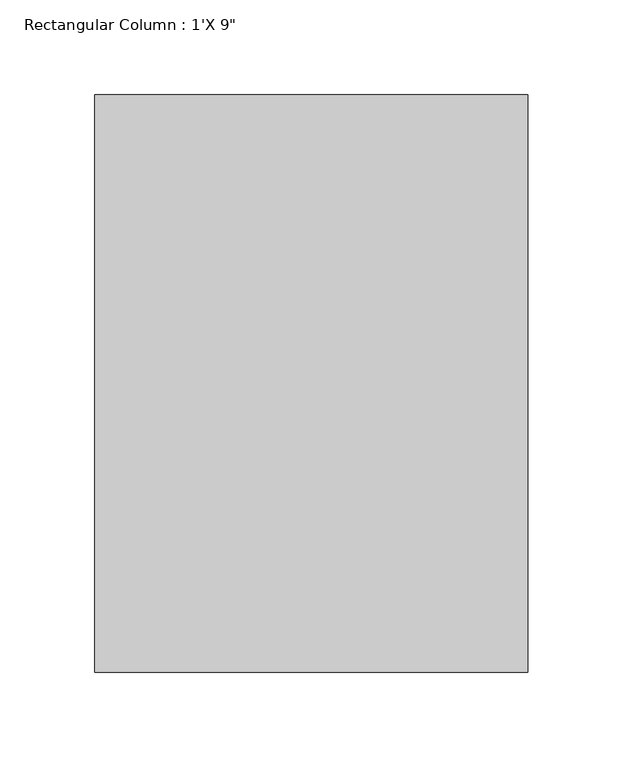
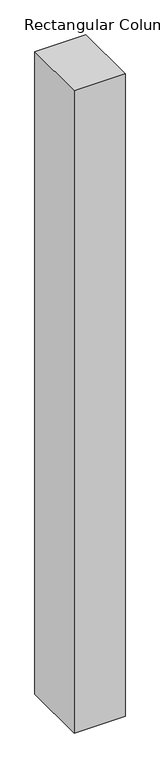
"""IFC4 building model written with IfcOpenShell, lengths in millimetres: column geometry."""

from ifc_helpers import new_model, si_unit, frame, origin, place, context, project, spatial, polyline, outline, extrude, source, transform, mapped, element, save


def column_1c121444(model_context):
    return source(origin(), model_context, "Body", "SweptSolid", [
        extrude(outline(polyline([(114.3, 152.4), (114.3, -152.4), (-114.3, -152.4), (-114.3, 152.4), (114.3, 152.4)])), frame((0.0, 0.0, 22402.8), z_axis=(0.0, 0.0, 1.0), x_axis=(1.0, 0.0, 0.0)), (0.0, 0.0, 1.0), 3048.0),
    ])


if __name__ == "__main__":
    model = new_model("IFC4")
    model_context = context("Model", 3, world=origin())
    ifc_project = project(units=[si_unit("LENGTHUNIT", "METRE", prefix="MILLI")], contexts=[model_context])
    site = spatial("IfcSite", under=ifc_project)
    building = spatial("IfcBuilding", under=site)
    placement = place(None, origin())
    column_shape = column_1c121444(model_context)
    element("IfcColumn", 1, ObjectType="Rectangular Column : 1'X 9\"", at=placement, inside=building, context=model_context, shape_type="MappedRepresentation", body=[
        mapped(column_shape, transform((0.0, 0.0, 0.0), x_axis=(1.0, 0.0, 0.0), y_axis=(0.0, 1.0, 0.0), z_axis=(0.0, 0.0, 1.0))),
    ])
    save(model, "model.ifc")

# Revit data of these elements
# Type "Rectangular Column : 1'X 9\""
#   Assembly Code = "B1010200"
#   Depth = 1' - 0"
#   Offset Base = 0' - 0"
#   Offset Top = 0' - 0"
#   Width = 0' - 9"
#   Material = none
